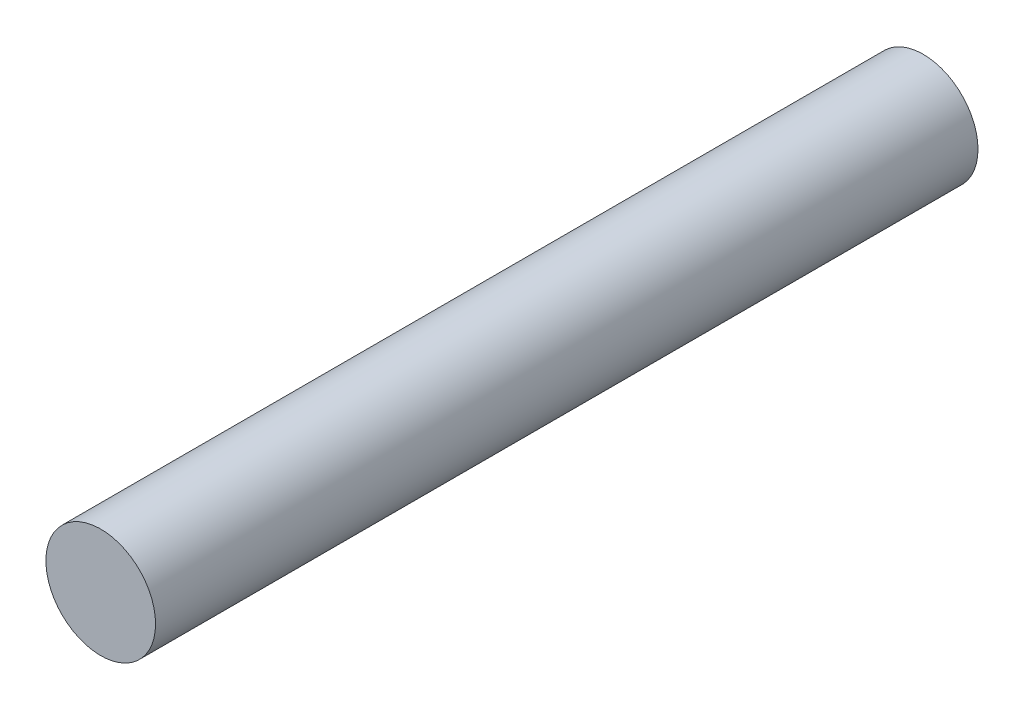
from build123d import *

# Parameters (mm, degrees)
PIN_PROFILE_4_R     = 2
PIN_BODY_4X30_DEPTH = 30


with BuildPart() as part:
    # Pin Profile Ø4 → Pin Body Ø4x30 (new body)
    with BuildSketch(Plane.XY):
        Circle(PIN_PROFILE_4_R)
    extrude(amount=PIN_BODY_4X30_DEPTH)


solid = part.part
